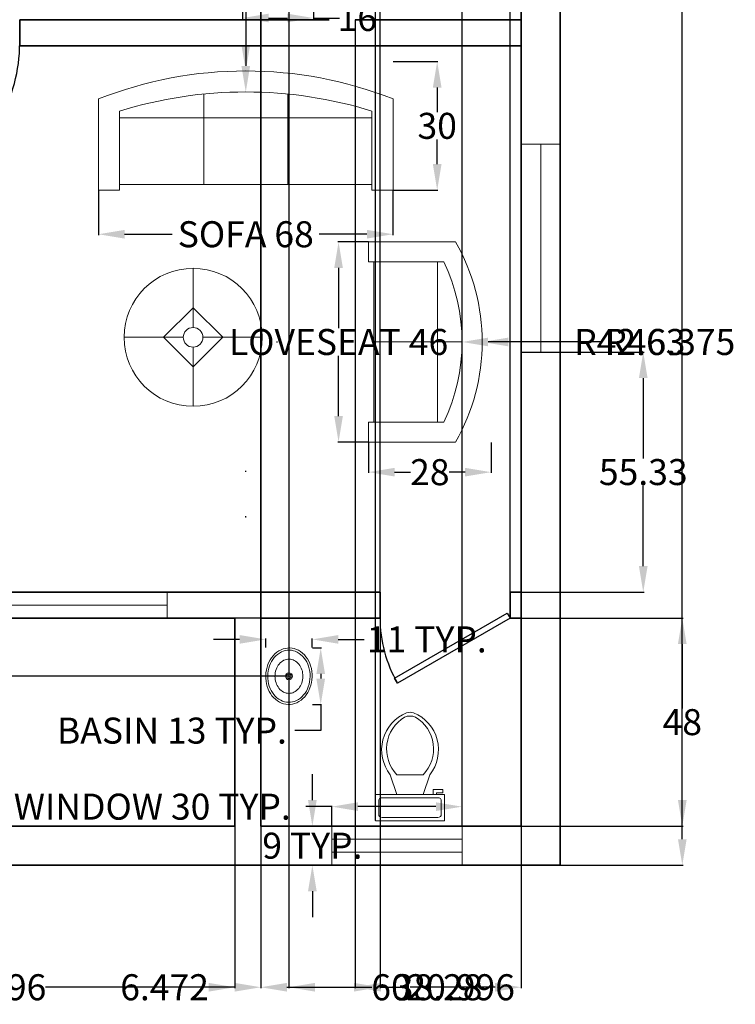
# Model space of a CAD drawing. Units: inches. Extents: x 351 to 774, y 111 to 703.
# Tile 3 of 6: x 608 to 773, y 111 to 338. Entities that reach past the tile are written whole.
import ezdxf

# ---------------------------------------------------------------- set-up
doc = ezdxf.new("R2010")
doc.units = ezdxf.units.IN
doc.header["$MEASUREMENT"] = 0
for name, color, linetype, lineweight in [('A-ANNO-DIMS', 2, 'Continuous', 18), ('A-DOOR', 3, 'Continuous', 25), ('A-FLOR-FIXT', 9, 'Continuous', 18), ('A-FURN', 8, 'Continuous', 18), ('A-GLAZ', 4, 'Continuous', 18), ('A-WALL', 7, 'Continuous', 35)]:
    doc.layers.add(name, color=color, linetype=linetype, lineweight=lineweight)
doc.styles.get("Standard").update_dxf_attribs({"font": 'arial.ttf'})
doc.dimstyles.get("Standard").update_dxf_attribs({"dimtxt": 6, "dimasz": 6, "dimexe": 0.18, "dimexo": 0.0625, "dimgap": 0.09, "dimtad": 0, "dimtih": 1, "dimtoh": 1, "dimdec": 0, "dimzin": 0, "dimdsep": 46, "dimlunit": 3, "dimtxsty": 'Standard', "dimcen": 0.09, "dimadec": 0, "dimazin": 0, "dimtfac": 1, "dimtdec": 0, "dimtofl": 0, "dimtmove": 0, "dimatfit": 3, "dimfxl": 1, "dimtolj": 1, "dimtzin": 0, "dimarcsym": 0})

# ---------------------------------------------------------------- blocks, each defined once
blk = doc.blocks.new('*U2')
for p, q in [((-40, 0), (-40, 6)), ((0, 0), (0, 6))]:
    blk.add_line(p, q)
blk.add_lwpolyline([(0, 0), (-34.64, -20), (-35.52, -18.48), (-0.88, 1.52)], close=True)
blk.add_arc((0, 0), 40, 180, 210)
blk = doc.blocks.new('*U5')
for p, q in [((0, 0), (0, 6)), ((40, 0), (40, 6))]:
    blk.add_line(p, q)
blk.add_lwpolyline([(0, 0), (34.64, -20), (35.52, -18.48), (0.88, 1.52)], close=True)
blk.add_arc((0, 0), 40, 330, 0)
blk = doc.blocks.new('Lamp - Table')
for p, q in [((0, 7), (0, 1)), ((0, 3), (-3, 0)), ((3, 0), (0, 3)), ((-1, 0), (-7, 0)), ((-3, 0), (0, -3)), ((0, -3), (3, 0)), ((1, 0), (7, 0)), ((0, -1), (0, -7))]:
    blk.add_line(p, q)
for radius in [7, 1]:
    blk.add_circle((0, 0), radius)
blk = doc.blocks.new('Sink - Oval top')
for p, q in [((-1, 0), (1, 0)), ((0, 1), (0, -1))]:
    blk.add_line(p, q)
for points in [[(-12.23, 0.39, 0.117634), (-11.46, -3.36, 0.104469), (-8.88, -6.8, 0.090016), (-5.08, -9.07, 0.08192), (-0.32, -10.02, 0.08192), (4.49, -9.38, 0.090016), (8.42, -7.36, 0.104469), (11.22, -4.09, 0.117634), (12.23, -0.39, 0.117634), (11.46, 3.36, 0.104469), (8.88, 6.8, 0.090016), (5.08, 9.07, 0.08192), (0.32, 10.02, 0.08192), (-4.49, 9.38, 0.090016), (-8.42, 7.36, 0.104469), (-11.22, 4.09, 0.117634)], [(-11.29, 0.16, 0.118622), (-10.52, -3.25, 0.104678), (-8.07, -6.36, 0.089562), (-4.54, -8.37, 0.081185), (-0.13, -9.15, 0.081185), (4.3, -8.49, 0.089562), (7.89, -6.58, 0.104678), (10.42, -3.55, 0.118622), (11.29, -0.16, 0.118622), (10.52, 3.25, 0.104678), (8.07, 6.36, 0.089562), (4.54, 8.37, 0.081185), (0.13, 9.15, 0.081185), (-4.3, 8.49, 0.089562), (-7.89, 6.58, 0.104678), (-10.42, 3.55, 0.118622)], [(-7.42, 0.08, 0.118283), (-6.91, -2.17, 0.104607), (-5.29, -4.21, 0.089718), (-2.97, -5.53, 0.081436), (-0.07, -6.04, 0.081436), (2.84, -5.59, 0.089718), (5.2, -4.33, 0.104607), (6.86, -2.32, 0.118283), (7.42, -0.08, 0.118283), (6.91, 2.17, 0.104607), (5.29, 4.21, 0.089718), (2.97, 5.53, 0.081436), (0.07, 6.04, 0.081436), (-2.84, 5.59, 0.089718), (-5.2, 4.33, 0.104607), (-6.86, 2.32, 0.118283)]]:
    blk.add_lwpolyline(points, format="xyb", close=True)
for radius in [1.5, 1]:
    blk.add_circle((0, 0), radius)
blk = doc.blocks.new('Sofa - Roundback 7 ft.')
for p, q in [((-12.00002, -32.4421), (-12.00003, -6.5971)), ((11.99997, -32.4421), (11.99998, -6.5971)), ((-36.000027, -34), (-36.000027, -11.4696)), ((-35.999844, -13.3819), (35.9998, -13.3819)), ((35.99998, -34), (35.99998, -11.4696)), ((-36.000027, -32.4421), (35.99998, -32.4421))]:
    blk.add_line(p, q)
for points in [[(-36.000027, -34), (-42.000027, -34), (-42.000027, -8)], [(41.99998, -8), (41.99998, -34), (35.99998, -34)]]:
    blk.add_lwpolyline(points)
for centre, radius, start, end in [((0, -114.25), 114.25, 68.43141, 111.5686), ((-0.00001, -127.1968), 121.1968, 72.72033, 107.2797)]:
    blk.add_arc(centre, radius, start, end)
blk = doc.blocks.new('Sofa - Roundback Loveseat 5 ft.')
for p, q in [((0, -32.44198), (0, -5.99998)), ((-24, -33.99998), (-24, -11.46958)), ((24.00004, -33.99998), (24.00004, -11.46958)), ((-23.9998, -13.38178), (23.99986, -13.38178)), ((-24, -32.44198), (24.00004, -32.44198))]:
    blk.add_line(p, q)
for points in [[(-24, -33.99998), (-30, -33.99998), (-30, -7.99998)], [(30.00004, -7.99998), (30.00004, -33.99998), (24.00004, -33.99998)]]:
    blk.add_lwpolyline(points)
for centre, radius, start, end in [((0, -60.24998), 60.24998, 60.13715, 119.8628), ((0, -61.38438), 55.38444, 64.32083, 115.6792)]:
    blk.add_arc(centre, radius, start, end)
blk = doc.blocks.new('Toilet - top')
for p, q in [((9.5, -6), (9.5, -2)), ((-10, -8.5), (-8, -8.5)), ((-10, -9.5), (-10, -8.5)), ((-8, -8.5), (-8, -8)), ((-7, -8), (-7, -9.5)), ((-4, -8), (-6, -14)), ((4, -8), (6, -14)), ((-7, -9.5), (-10, -9.5)), ((4, -14), (-4, -14))]:
    blk.add_line(p, q)
blk.add_lwpolyline([(10.5, -8), (10.5, 0), (-10.5, 0), (-10.5, -8)], close=True)
for points in [[(-9.5, -2), (-9.5, -6)], [(8.5, -1), (-8.5, -1)], [(-8.5, -7), (8.5, -7)]]:
    blk.add_lwpolyline(points)
for centre, radius, start, end in [((-8.62, -1.88), 0.884, 81.8699, 188.1301), ((8.62, -1.88), 0.884, 351.8699, 98.1301), ((-8.62, -6.12), 0.884, 171.8699, 278.1301), ((8.62, -6.12), 0.884, 261.8699, 8.1301), ((3.52, -21.58), 12.17, 141.4691, 247.9714), ((4.2, -21.82), 11.33, 136.3677, 238.9468), ((-3.52, -21.58), 12.17, 292.0284, 38.5307), ((-4.2, -21.82), 11.33, 301.053, 43.6321), ((0, -27.88), 4, 245.7318, 294.2682), ((0, -29), 4, 254.8605, 285.1395)]:
    blk.add_arc(centre, radius, start, end)
blk = doc.blocks.new('WIN-48IN-6IN-WALL')
blk.add_line((3, 48), (3, 0))
blk.add_lwpolyline([(0, 48), (6, 48), (6, 0), (0, 0)], close=True)
blk = doc.blocks.new('WIN-48IN-9IN-WALL')
blk.add_line((4.5, 48), (4.5, 0))
blk.add_lwpolyline([(0, 0), (9, 0), (9, 48), (0, 48)], close=True)
blk = doc.blocks.new('WIN-BATH-30IN-9IN-WALL')
for p, q in [((0, 0), (0, 9)), ((0, 9), (30, 9)), ((30, 9), (30, 0)), ((0, 6), (30, 6)), ((30, 3), (0, 3)), ((30, 0), (0, 0))]:
    blk.add_line(p, q)
blk = doc.blocks.new('*D26')
at = {"layer": 'A-ANNO-DIMS', "color": 0, "lineweight": -2, "transparency": 16777216}
for p, q in [((680.41, 156.74), (674.41, 156.74)), ((680.41, 152.3), (680.41, 156.92)), ((704.41, 156.74), (686.41, 156.74)), ((710.41, 152.3), (710.41, 156.92))]:
    blk.add_line(p, q, dxfattribs=at)
at = {"layer": 'A-ANNO-DIMS', "color": 0, "transparency": 16777216}
for points in [[(686.41, 157.74), (686.41, 155.74), (680.41, 156.74)], [(704.41, 157.74), (704.41, 155.74), (710.41, 156.74)]]:
    blk.add_solid(points, dxfattribs=at)
at = {"layer": 'Defpoints', "color": 0, "transparency": 16777216}
for p in [(680.41, 156.74), (680.41, 152.24), (710.41, 152.24)]:
    blk.add_point(p, dxfattribs=at)
at = {"layer": 'A-ANNO-DIMS', "color": 0, "transparency": 16777216, "insert": (631.89, 156.74), "char_height": 6, "attachment_point": 5}
blk.add_mtext('\\A1;WC WINDOW 30 TYP.', dxfattribs=at)
blk = doc.blocks.new('*D27')
at = {"layer": 'A-ANNO-DIMS', "color": 0, "lineweight": -2, "transparency": 16777216}
for p, q in [((675.91, 158.24), (675.91, 164.24)), ((680.35, 152.24), (675.73, 152.24)), ((680.35, 143.24), (675.73, 143.24)), ((675.91, 137.24), (675.91, 131.24))]:
    blk.add_line(p, q, dxfattribs=at)
at = {"layer": 'A-ANNO-DIMS', "color": 0, "transparency": 16777216}
for points in [[(674.91, 158.24), (676.91, 158.24), (675.91, 152.24)], [(674.91, 137.24), (676.91, 137.24), (675.91, 143.24)]]:
    blk.add_solid(points, dxfattribs=at)
at = {"layer": 'Defpoints', "color": 0, "transparency": 16777216}
for p in [(680.41, 152.24), (675.91, 143.24), (680.41, 143.24)]:
    blk.add_point(p, dxfattribs=at)
at = {"layer": 'A-ANNO-DIMS', "color": 0, "transparency": 16777216, "insert": (675.91, 147.74), "char_height": 6, "attachment_point": 5}
blk.add_mtext('\\A1;9 TYP.', dxfattribs=at)
blk = doc.blocks.new('*D30')
at = {"layer": 'A-ANNO-DIMS', "color": 0, "lineweight": -2, "transparency": 16777216}
for p, q in [((675.94, 193.36), (678.02, 193.36)), ((677.84, 187.36), (677.84, 186.28)), ((675.94, 180.28), (678.02, 180.28)), ((677.84, 180.28), (677.84, 174.28)), ((677.84, 174.28), (671.84, 174.28))]:
    blk.add_line(p, q, dxfattribs=at)
at = {"layer": 'A-ANNO-DIMS', "color": 0, "transparency": 16777216}
for points in [[(676.84, 187.36), (678.84, 187.36), (677.84, 193.36)], [(676.84, 186.28), (678.84, 186.28), (677.84, 180.28)]]:
    blk.add_solid(points, dxfattribs=at)
at = {"layer": 'Defpoints', "color": 0, "transparency": 16777216}
for p in [(675.88, 193.36), (675.88, 180.28), (677.84, 180.28)]:
    blk.add_point(p, dxfattribs=at)
at = {"layer": 'A-ANNO-DIMS', "color": 0, "transparency": 16777216, "insert": (643.54, 174.28), "char_height": 6, "attachment_point": 5}
blk.add_mtext('\\A1;BASIN 13 TYP.', dxfattribs=at)
blk = doc.blocks.new('*D31')
at = {"layer": 'A-ANNO-DIMS', "color": 0, "lineweight": -2, "transparency": 16777216}
for p, q in [((659.15, 195.32), (653.15, 195.32)), ((665.15, 193.42), (665.15, 195.5)), ((675.88, 193.42), (675.88, 195.5)), ((681.88, 195.32), (687.88, 195.32))]:
    blk.add_line(p, q, dxfattribs=at)
at = {"layer": 'A-ANNO-DIMS', "color": 0, "transparency": 16777216}
for points in [[(659.15, 196.32), (659.15, 194.32), (665.15, 195.32)], [(681.88, 196.32), (681.88, 194.32), (675.88, 195.32)]]:
    blk.add_solid(points, dxfattribs=at)
at = {"layer": 'Defpoints', "color": 0, "transparency": 16777216}
for p in [(675.88, 195.32), (665.15, 193.36), (675.88, 193.36)]:
    blk.add_point(p, dxfattribs=at)
at = {"layer": 'A-ANNO-DIMS', "color": 0, "transparency": 16777216, "insert": (702.29, 195.32), "char_height": 6, "attachment_point": 5}
blk.add_mtext('\\A1;11 TYP.', dxfattribs=at)
blk = doc.blocks.new('*D39')
at = {"layer": 'A-ANNO-DIMS', "color": 0, "lineweight": -2, "transparency": 16777216}
for p, q in [((659.83, 342.77), (659.83, 338.45)), ((676.17, 342.77), (676.17, 338.45)), ((665.83, 338.63), (670.17, 338.63)), ((676.17, 338.63), (682.17, 338.63))]:
    blk.add_line(p, q, dxfattribs=at)
at = {"layer": 'A-ANNO-DIMS', "color": 0, "transparency": 16777216}
for points in [[(665.83, 339.63), (665.83, 337.63), (659.83, 338.63)], [(670.17, 339.63), (670.17, 337.63), (676.17, 338.63)]]:
    blk.add_solid(points, dxfattribs=at)
at = {"layer": 'Defpoints', "color": 0, "transparency": 16777216}
for p in [(659.83, 342.83), (676.17, 342.83), (676.17, 338.63)]:
    blk.add_point(p, dxfattribs=at)
at = {"layer": 'A-ANNO-DIMS', "color": 0, "transparency": 16777216, "insert": (686.27, 338.63), "char_height": 6, "attachment_point": 5}
blk.add_mtext('\\A1;16', dxfattribs=at)
blk = doc.blocks.new('*D40')
at = {"layer": 'A-ANNO-DIMS', "color": 0, "lineweight": -2, "transparency": 16777216}
for p, q in [((626.61, 298.88), (626.61, 288.58)), ((694.5, 298.88), (694.5, 288.58)), ((632.61, 288.76), (643.6, 288.76)), ((688.5, 288.76), (677.51, 288.76))]:
    blk.add_line(p, q, dxfattribs=at)
at = {"layer": 'A-ANNO-DIMS', "color": 0, "transparency": 16777216}
for points in [[(632.61, 289.76), (632.61, 287.76), (626.61, 288.76)], [(688.5, 289.76), (688.5, 287.76), (694.5, 288.76)]]:
    blk.add_solid(points, dxfattribs=at)
at = {"layer": 'Defpoints', "color": 0, "transparency": 16777216}
for p in [(626.61, 298.94), (694.5, 298.94), (694.5, 288.76)]:
    blk.add_point(p, dxfattribs=at)
at = {"layer": 'A-ANNO-DIMS', "color": 0, "transparency": 16777216, "insert": (660.56, 288.76), "char_height": 6, "attachment_point": 5}
blk.add_mtext('\\A1;SOFA 68', dxfattribs=at)
blk = doc.blocks.new('*D41')
at = {"layer": 'A-ANNO-DIMS', "color": 0, "lineweight": -2, "transparency": 16777216}
for p, q in [((694.57, 328.58), (704.87, 328.58)), ((704.69, 322.58), (704.69, 316.92)), ((704.69, 304.94), (704.69, 310.61)), ((694.57, 298.94), (704.87, 298.94))]:
    blk.add_line(p, q, dxfattribs=at)
at = {"layer": 'A-ANNO-DIMS', "color": 0, "transparency": 16777216}
for points in [[(703.69, 322.58), (705.69, 322.58), (704.69, 328.58)], [(703.69, 304.94), (705.69, 304.94), (704.69, 298.94)]]:
    blk.add_solid(points, dxfattribs=at)
at = {"layer": 'Defpoints', "color": 0, "transparency": 16777216}
for p in [(694.5, 328.58), (704.69, 328.58), (694.5, 298.94)]:
    blk.add_point(p, dxfattribs=at)
at = {"layer": 'A-ANNO-DIMS', "color": 0, "transparency": 16777216, "insert": (704.69, 313.76), "char_height": 6, "attachment_point": 5}
blk.add_mtext('\\A1;30', dxfattribs=at)
blk = doc.blocks.new('*D42')
at = {"layer": 'A-ANNO-DIMS', "color": 0, "lineweight": -2, "transparency": 16777216}
for p, q in [((688.82, 287), (681.77, 287)), ((681.95, 281), (681.95, 267.1)), ((681.95, 246.82), (681.95, 260.71)), ((688.82, 240.82), (681.77, 240.82))]:
    blk.add_line(p, q, dxfattribs=at)
at = {"layer": 'A-ANNO-DIMS', "color": 0, "transparency": 16777216}
for points in [[(680.95, 281), (682.95, 281), (681.95, 287)], [(680.95, 246.82), (682.95, 246.82), (681.95, 240.82)]]:
    blk.add_solid(points, dxfattribs=at)
at = {"layer": 'Defpoints', "color": 0, "transparency": 16777216}
for p in [(688.88, 287), (681.95, 240.82), (688.88, 240.82)]:
    blk.add_point(p, dxfattribs=at)
at = {"layer": 'A-ANNO-DIMS', "color": 0, "transparency": 16777216, "insert": (681.95, 263.91), "char_height": 6, "attachment_point": 5}
blk.add_mtext('\\A1;LOVESEAT 46', dxfattribs=at)
blk = doc.blocks.new('*D43')
at = {"layer": 'A-ANNO-DIMS', "color": 0, "lineweight": -2, "transparency": 16777216}
for p, q in [((688.88, 240.75), (688.88, 233.71)), ((717.1, 240.75), (717.1, 233.71)), ((694.88, 233.89), (698.55, 233.89)), ((711.1, 233.89), (707.44, 233.89))]:
    blk.add_line(p, q, dxfattribs=at)
at = {"layer": 'A-ANNO-DIMS', "color": 0, "transparency": 16777216}
for points in [[(694.88, 234.89), (694.88, 232.89), (688.88, 233.89)], [(711.1, 234.89), (711.1, 232.89), (717.1, 233.89)]]:
    blk.add_solid(points, dxfattribs=at)
at = {"layer": 'Defpoints', "color": 0, "transparency": 16777216}
for p in [(688.88, 240.82), (717.1, 240.82), (717.1, 233.89)]:
    blk.add_point(p, dxfattribs=at)
at = {"layer": 'A-ANNO-DIMS', "color": 0, "transparency": 16777216, "insert": (702.99, 233.89), "char_height": 6, "attachment_point": 5}
blk.add_mtext('\\A1;28', dxfattribs=at)
blk = doc.blocks.new('*D47')
at = {"layer": 'A-ANNO-DIMS', "color": 0, "lineweight": -2, "transparency": 16777216}
for p, q in [((733.11, 671.24), (761.37, 671.24)), ((761.19, 665.24), (761.19, 410.4)), ((761.19, 149.24), (761.19, 404.09)), ((733.11, 143.24), (761.37, 143.24))]:
    blk.add_line(p, q, dxfattribs=at)
at = {"layer": 'A-ANNO-DIMS', "color": 0, "transparency": 16777216}
for points in [[(760.19, 665.24), (762.19, 665.24), (761.19, 671.24)], [(760.19, 149.24), (762.19, 149.24), (761.19, 143.24)]]:
    blk.add_solid(points, dxfattribs=at)
at = {"layer": 'Defpoints', "color": 0, "transparency": 16777216}
for p in [(733.04, 671.24), (761.19, 671.24), (733.04, 143.24)]:
    blk.add_point(p, dxfattribs=at)
at = {"layer": 'A-ANNO-DIMS', "color": 0, "transparency": 16777216, "insert": (761.19, 407.24), "char_height": 6, "attachment_point": 5}
blk.add_mtext('\\A1;528', dxfattribs=at)
blk = doc.blocks.new('*D61')
at = {"layer": 'A-ANNO-DIMS', "color": 0, "lineweight": -2, "transparency": 16777216}
for p, q in [((562.04, 152.18), (562.04, 114.91)), ((658.04, 152.18), (658.04, 114.91)), ((568.04, 115.09), (605.66, 115.09)), ((652.04, 115.09), (614.43, 115.09))]:
    blk.add_line(p, q, dxfattribs=at)
at = {"layer": 'A-ANNO-DIMS', "color": 0, "transparency": 16777216}
for points in [[(568.04, 116.09), (568.04, 114.09), (562.04, 115.09)], [(652.04, 116.09), (652.04, 114.09), (658.04, 115.09)]]:
    blk.add_solid(points, dxfattribs=at)
at = {"layer": 'Defpoints', "color": 0, "transparency": 16777216}
for p in [(562.04, 152.24), (658.04, 152.24), (658.04, 115.09)]:
    blk.add_point(p, dxfattribs=at)
at = {"layer": 'A-ANNO-DIMS', "color": 0, "transparency": 16777216, "insert": (610.04, 115.09), "char_height": 6, "attachment_point": 5}
blk.add_mtext('\\A1;96', dxfattribs=at)
blk = doc.blocks.new('*D62')
at = {"layer": 'A-ANNO-DIMS', "color": 0, "lineweight": -2, "transparency": 16777216}
for p, q in [((664.04, 152.18), (664.04, 114.91)), ((724.04, 152.18), (724.04, 114.91)), ((670.04, 115.09), (689.65, 115.09)), ((718.04, 115.09), (698.44, 115.09))]:
    blk.add_line(p, q, dxfattribs=at)
at = {"layer": 'A-ANNO-DIMS', "color": 0, "transparency": 16777216}
for points in [[(670.04, 116.09), (670.04, 114.09), (664.04, 115.09)], [(718.04, 116.09), (718.04, 114.09), (724.04, 115.09)]]:
    blk.add_solid(points, dxfattribs=at)
at = {"layer": 'Defpoints', "color": 0, "transparency": 16777216}
for p in [(664.04, 152.24), (724.04, 152.24), (724.04, 115.09)]:
    blk.add_point(p, dxfattribs=at)
at = {"layer": 'A-ANNO-DIMS', "color": 0, "transparency": 16777216, "insert": (694.04, 115.09), "char_height": 6, "attachment_point": 5}
blk.add_mtext('\\A1;60', dxfattribs=at)
blk = doc.blocks.new('*D63')
at = {"layer": 'A-ANNO-DIMS', "color": 0, "lineweight": -2, "transparency": 16777216}
for p, q in [((724.11, 200.24), (761.37, 200.24)), ((761.19, 194.24), (761.19, 179.4)), ((761.19, 158.24), (761.19, 173.09)), ((724.11, 152.24), (761.37, 152.24))]:
    blk.add_line(p, q, dxfattribs=at)
at = {"layer": 'A-ANNO-DIMS', "color": 0, "transparency": 16777216}
for points in [[(760.19, 194.24), (762.19, 194.24), (761.19, 200.24)], [(760.19, 158.24), (762.19, 158.24), (761.19, 152.24)]]:
    blk.add_solid(points, dxfattribs=at)
at = {"layer": 'Defpoints', "color": 0, "transparency": 16777216}
for p in [(724.04, 200.24), (761.19, 200.24), (724.04, 152.24)]:
    blk.add_point(p, dxfattribs=at)
at = {"layer": 'A-ANNO-DIMS', "color": 0, "transparency": 16777216, "insert": (761.19, 176.24), "char_height": 6, "attachment_point": 5}
blk.add_mtext('\\A1;48', dxfattribs=at)
blk = doc.blocks.new('*D67')
at = {"layer": 'A-ANNO-DIMS', "color": 0, "lineweight": -2, "transparency": 16777216}
for p, q in [((724.11, 261.57), (752.37, 261.57)), ((752.19, 255.57), (752.19, 237.06)), ((752.19, 212.24), (752.19, 230.75)), ((724.11, 206.24), (752.37, 206.24))]:
    blk.add_line(p, q, dxfattribs=at)
at = {"layer": 'A-ANNO-DIMS', "color": 0, "transparency": 16777216}
for points in [[(751.19, 255.57), (753.19, 255.57), (752.19, 261.57)], [(751.19, 212.24), (753.19, 212.24), (752.19, 206.24)]]:
    blk.add_solid(points, dxfattribs=at)
at = {"layer": 'Defpoints', "color": 0, "transparency": 16777216}
for p in [(724.04, 261.57), (724.04, 206.24), (752.19, 206.24)]:
    blk.add_point(p, dxfattribs=at)
at = {"layer": 'A-ANNO-DIMS', "color": 0, "transparency": 16777216, "insert": (752.19, 233.91), "char_height": 6, "attachment_point": 5}
blk.add_mtext('\\A1;55.33', dxfattribs=at)
blk = doc.blocks.new('*D68')
at = {"layer": 'A-ANNO-DIMS', "color": 0, "lineweight": -2, "transparency": 16777216}
for p, q in [((685.77, 338.18), (685.77, 114.91)), ((724.04, 338.18), (724.04, 114.91)), ((691.77, 115.09), (694.69, 115.09)), ((718.04, 115.09), (715.12, 115.09))]:
    blk.add_line(p, q, dxfattribs=at)
at = {"layer": 'A-ANNO-DIMS', "color": 0, "transparency": 16777216}
for points in [[(691.77, 116.09), (691.77, 114.09), (685.77, 115.09)], [(718.04, 116.09), (718.04, 114.09), (724.04, 115.09)]]:
    blk.add_solid(points, dxfattribs=at)
at = {"layer": 'Defpoints', "color": 0, "transparency": 16777216}
for p in [(685.77, 338.24), (724.04, 338.24), (724.04, 115.09)]:
    blk.add_point(p, dxfattribs=at)
at = {"layer": 'A-ANNO-DIMS', "color": 0, "transparency": 16777216, "insert": (704.9, 115.09), "char_height": 6, "attachment_point": 5}
blk.add_mtext('\\A1;38.28', dxfattribs=at)
blk = doc.blocks.new('*D69')
at = {"layer": 'A-ANNO-DIMS', "color": 0, "lineweight": -2, "transparency": 16777216}
for p, q in [((724.04, 473.44), (724.04, 114.91)), ((664.04, 470.18), (664.04, 114.91)), ((670.04, 115.09), (689.65, 115.09)), ((718.04, 115.09), (698.44, 115.09))]:
    blk.add_line(p, q, dxfattribs=at)
at = {"layer": 'A-ANNO-DIMS', "color": 0, "transparency": 16777216}
for points in [[(670.04, 116.09), (670.04, 114.09), (664.04, 115.09)], [(718.04, 116.09), (718.04, 114.09), (724.04, 115.09)]]:
    blk.add_solid(points, dxfattribs=at)
at = {"layer": 'Defpoints', "color": 0, "transparency": 16777216}
for p in [(724.04, 473.5), (664.04, 470.24), (724.04, 115.09)]:
    blk.add_point(p, dxfattribs=at)
at = {"layer": 'A-ANNO-DIMS', "color": 0, "transparency": 16777216, "insert": (694.04, 115.09), "char_height": 6, "attachment_point": 5}
blk.add_mtext('\\A1;60', dxfattribs=at)
blk = doc.blocks.new('*D86')
at = {"layer": 'A-ANNO-DIMS', "color": 0, "lineweight": -2, "transparency": 16777216}
for p, q in [((710.41, 152.3), (710.41, 699.57)), ((724.04, 152.3), (724.04, 699.57)), ((716.41, 699.39), (718.04, 699.39)), ((724.04, 699.39), (730.04, 699.39))]:
    blk.add_line(p, q, dxfattribs=at)
at = {"layer": 'A-ANNO-DIMS', "color": 0, "transparency": 16777216}
for points in [[(716.41, 700.39), (716.41, 698.39), (710.41, 699.39)], [(718.04, 700.39), (718.04, 698.39), (724.04, 699.39)]]:
    blk.add_solid(points, dxfattribs=at)
at = {"layer": 'Defpoints', "color": 0, "transparency": 16777216}
for p in [(724.04, 699.39), (710.41, 152.24), (724.04, 152.24)]:
    blk.add_point(p, dxfattribs=at)
at = {"layer": 'A-ANNO-DIMS', "color": 0, "transparency": 16777216, "insert": (742.3, 699.39), "char_height": 6, "attachment_point": 5}
blk.add_mtext('\\A1;13.633', dxfattribs=at)
blk = doc.blocks.new('*D87')
at = {"layer": 'A-ANNO-DIMS', "color": 0, "lineweight": -2, "transparency": 16777216}
for p, q in [((691.51, 206.3), (691.51, 699.57)), ((721.51, 206.3), (721.51, 699.57)), ((697.51, 699.39), (702.14, 699.39)), ((715.51, 699.39), (710.89, 699.39))]:
    blk.add_line(p, q, dxfattribs=at)
at = {"layer": 'A-ANNO-DIMS', "color": 0, "transparency": 16777216}
for points in [[(697.51, 700.39), (697.51, 698.39), (691.51, 699.39)], [(715.51, 700.39), (715.51, 698.39), (721.51, 699.39)]]:
    blk.add_solid(points, dxfattribs=at)
at = {"layer": 'Defpoints', "color": 0, "transparency": 16777216}
for p in [(721.51, 699.39), (691.51, 206.24), (721.51, 206.24)]:
    blk.add_point(p, dxfattribs=at)
at = {"layer": 'A-ANNO-DIMS', "color": 0, "transparency": 16777216, "insert": (706.51, 699.39), "char_height": 6, "attachment_point": 5}
blk.add_mtext('\\A1;30', dxfattribs=at)
blk = doc.blocks.new('*D88')
at = {"layer": 'A-ANNO-DIMS', "color": 0, "lineweight": -2, "transparency": 16777216}
for p, q in [((664.043027, 200.304576), (664.043027, 699.572076)), ((691.510725, 200.304576), (691.510725, 699.572076)), ((658.043027, 699.392076), (652.043027, 699.392076)), ((697.510725, 699.392076), (703.510725, 699.392076))]:
    blk.add_line(p, q, dxfattribs=at)
at = {"layer": 'A-ANNO-DIMS', "color": 0, "transparency": 16777216}
for points in [[(658.043027, 700.392076), (658.043027, 698.392076), (664.043027, 699.392076)], [(697.510725, 700.392076), (697.510725, 698.392076), (691.510725, 699.392076)]]:
    blk.add_solid(points, dxfattribs=at)
at = {"layer": 'Defpoints', "color": 0, "transparency": 16777216}
for p in [(691.510725, 699.392076), (664.043027, 200.242076), (691.510725, 200.242076)]:
    blk.add_point(p, dxfattribs=at)
at = {"layer": 'A-ANNO-DIMS', "color": 0, "transparency": 16777216, "insert": (677.776876, 699.392076), "char_height": 6, "attachment_point": 5}
blk.add_mtext('\\A1;27.47', dxfattribs=at)
blk = doc.blocks.new('*D101')
at = {"layer": 'A-ANNO-DIMS', "color": 0, "lineweight": -2, "transparency": 16777216}
for p, q in [((664.04, 152.3), (664.04, 699.57)), ((690.48, 153.55), (690.48, 699.57)), ((658.04, 699.39), (652.04, 699.39)), ((696.48, 699.39), (702.48, 699.39))]:
    blk.add_line(p, q, dxfattribs=at)
at = {"layer": 'A-ANNO-DIMS', "color": 0, "transparency": 16777216}
for points in [[(658.04, 700.39), (658.04, 698.39), (664.04, 699.39)], [(696.48, 700.39), (696.48, 698.39), (690.48, 699.39)]]:
    blk.add_solid(points, dxfattribs=at)
at = {"layer": 'Defpoints', "color": 0, "transparency": 16777216}
for p in [(664.04, 699.39), (664.04, 152.24), (690.48, 153.49)]:
    blk.add_point(p, dxfattribs=at)
at = {"layer": 'A-ANNO-DIMS', "color": 0, "transparency": 16777216, "insert": (677.26, 699.39), "char_height": 6, "attachment_point": 5}
blk.add_mtext('\\A1;26.433', dxfattribs=at)
blk = doc.blocks.new('*D102')
at = {"layer": 'A-ANNO-DIMS', "color": 0, "lineweight": -2, "transparency": 16777216}
for p, q in [((392.89, 200.24), (392.89, 206.24)), ((392.89, 206.24), (398.89, 206.24)), ((663.98, 200.24), (392.71, 200.24)), ((392.89, 192.82), (392.89, 194.24)), ((670.45, 186.82), (392.71, 186.82))]:
    blk.add_line(p, q, dxfattribs=at)
at = {"layer": 'A-ANNO-DIMS', "color": 0, "transparency": 16777216}
for points in [[(391.89, 194.24), (393.89, 194.24), (392.89, 200.24)], [(391.89, 192.82), (393.89, 192.82), (392.89, 186.82)]]:
    blk.add_solid(points, dxfattribs=at)
at = {"layer": 'Defpoints', "color": 0, "transparency": 16777216}
for p in [(392.89, 200.24), (664.04, 200.24), (670.51, 186.82)]:
    blk.add_point(p, dxfattribs=at)
at = {"layer": 'A-ANNO-DIMS', "color": 0, "transparency": 16777216, "insert": (411.14, 206.24), "char_height": 6, "attachment_point": 5}
blk.add_mtext('\\A1;13.424', dxfattribs=at)
blk = doc.blocks.new('*D108')
at = {"layer": 'A-ANNO-DIMS', "color": 0, "lineweight": -2, "transparency": 16777216}
for p, q in [((664.04, 527.44), (664.04, 114.91)), ((670.51, 515.76), (670.51, 114.91)), ((658.04, 115.09), (652.04, 115.09)), ((676.51, 115.09), (682.51, 115.09))]:
    blk.add_line(p, q, dxfattribs=at)
at = {"layer": 'A-ANNO-DIMS', "color": 0, "transparency": 16777216}
for points in [[(658.04, 116.09), (658.04, 114.09), (664.04, 115.09)], [(676.51, 116.09), (676.51, 114.09), (670.51, 115.09)]]:
    blk.add_solid(points, dxfattribs=at)
at = {"layer": 'Defpoints', "color": 0, "transparency": 16777216}
for p in [(664.04, 527.5), (670.51, 515.82), (664.04, 115.09)]:
    blk.add_point(p, dxfattribs=at)
at = {"layer": 'A-ANNO-DIMS', "color": 0, "transparency": 16777216, "insert": (641.84, 115.09), "char_height": 6, "attachment_point": 5}
blk.add_mtext('\\A1;6.472', dxfattribs=at)
blk = doc.blocks.new('*D109')
at = {"layer": 'A-ANNO-DIMS', "color": 0, "lineweight": -2, "transparency": 16777216}
for p, q in [((691.51, 200.18), (691.51, 114.91)), ((670.51, 186.76), (670.51, 114.91)), ((676.51, 115.09), (685.51, 115.09)), ((691.51, 115.09), (697.51, 115.09))]:
    blk.add_line(p, q, dxfattribs=at)
at = {"layer": 'A-ANNO-DIMS', "color": 0, "transparency": 16777216}
for points in [[(676.51, 116.09), (676.51, 114.09), (670.51, 115.09)], [(685.51, 116.09), (685.51, 114.09), (691.51, 115.09)]]:
    blk.add_solid(points, dxfattribs=at)
at = {"layer": 'Defpoints', "color": 0, "transparency": 16777216}
for p in [(691.51, 200.24), (670.51, 186.82), (691.51, 115.09)]:
    blk.add_point(p, dxfattribs=at)
at = {"layer": 'A-ANNO-DIMS', "color": 0, "transparency": 16777216, "insert": (710.1, 115.09), "char_height": 6, "attachment_point": 5}
blk.add_mtext('\\A1;20.996', dxfattribs=at)
blk = doc.blocks.new('*D110')
at = {"layer": 'A-ANNO-DIMS', "color": 0, "lineweight": -2, "transparency": 16777216}
for p, q in [((666.56, 380.35), (660.56, 380.35)), ((660.56, 380.35), (660.56, 327.58)), ((660.47, 223.61), (660.65, 223.61)), ((660.56, 223.52), (660.56, 223.7))]:
    blk.add_line(p, q, dxfattribs=at)
at = {"layer": 'A-ANNO-DIMS', "color": 0, "transparency": 16777216}
blk.add_solid([(659.56, 327.58), (661.56, 327.58), (660.56, 321.58)], dxfattribs=at)
at = {"layer": 'Defpoints', "color": 0, "transparency": 16777216}
for p in [(660.56, 321.58), (660.56, 223.61)]:
    blk.add_point(p, dxfattribs=at)
at = {"layer": 'A-ANNO-DIMS', "color": 0, "transparency": 16777216, "insert": (679.64, 380.35), "char_height": 6, "attachment_point": 5}
blk.add_mtext('\\A1;R97.96', dxfattribs=at)
blk = doc.blocks.new('*D111')
at = {"layer": 'A-ANNO-DIMS', "color": 0, "lineweight": -2, "transparency": 16777216}
for p, q in [((666.56, 381.83), (660.56, 381.83)), ((660.56, 381.83), (660.56, 332.43)), ((660.47, 234.08), (660.65, 234.08)), ((660.56, 233.99), (660.56, 234.17))]:
    blk.add_line(p, q, dxfattribs=at)
at = {"layer": 'A-ANNO-DIMS', "color": 0, "transparency": 16777216}
blk.add_solid([(659.56, 332.43), (661.56, 332.43), (660.56, 326.43)], dxfattribs=at)
at = {"layer": 'Defpoints', "color": 0, "transparency": 16777216}
for p in [(660.56, 326.43), (660.56, 234.08)]:
    blk.add_point(p, dxfattribs=at)
at = {"layer": 'A-ANNO-DIMS', "color": 0, "transparency": 16777216, "insert": (679.66, 381.83), "char_height": 6, "attachment_point": 5}
blk.add_mtext('\\A1;R92.35', dxfattribs=at)
blk = doc.blocks.new('*D112')
at = {"layer": 'A-ANNO-DIMS', "color": 0, "lineweight": -2, "transparency": 16777216}
for p, q in [((668.59, 263.91), (668.77, 263.91)), ((668.68, 263.82), (668.68, 264)), ((742.88, 263.91), (721.05, 263.91))]:
    blk.add_line(p, q, dxfattribs=at)
at = {"layer": 'A-ANNO-DIMS', "color": 0, "transparency": 16777216}
blk.add_solid([(721.05, 264.91), (721.05, 262.91), (715.05, 263.91)], dxfattribs=at)
at = {"layer": 'Defpoints', "color": 0, "transparency": 16777216}
for p in [(668.68, 263.91), (715.05, 263.91)]:
    blk.add_point(p, dxfattribs=at)
at = {"layer": 'A-ANNO-DIMS', "color": 0, "transparency": 16777216, "insert": (758.31, 263.91), "char_height": 6, "attachment_point": 5}
blk.add_mtext('\\A1;R46.375', dxfattribs=at)
blk = doc.blocks.new('*D113')
at = {"layer": 'A-ANNO-DIMS', "color": 0, "lineweight": -2, "transparency": 16777216}
for p, q in [((667.71, 263.91), (667.89, 263.91)), ((667.8, 263.82), (667.8, 264)), ((736.01, 263.91), (716.43, 263.91))]:
    blk.add_line(p, q, dxfattribs=at)
at = {"layer": 'A-ANNO-DIMS', "color": 0, "transparency": 16777216}
blk.add_solid([(716.43, 264.91), (716.43, 262.91), (710.43, 263.91)], dxfattribs=at)
at = {"layer": 'Defpoints', "color": 0, "transparency": 16777216}
for p in [(667.8, 263.91), (710.43, 263.91)]:
    blk.add_point(p, dxfattribs=at)
at = {"layer": 'A-ANNO-DIMS', "color": 0, "transparency": 16777216, "insert": (749.1, 263.91), "char_height": 6, "attachment_point": 5}
blk.add_mtext('\\A1;R42.63', dxfattribs=at)

msp = doc.modelspace()

# ---------------------------------------------------------------- linework, layer by layer
at = {"layer": 'A-WALL'}
for p, q in [((608.4474, 332.2421), (608.4474, 338.2421)), ((679.7664, 338.2421), (608.4474, 338.2421)), ((724.043, 338.2421), (685.7664, 338.2421)), ((724.043, 332.2421), (608.4474, 332.2421)), ((724.043, 332.2421), (724.043, 206.2421)), ((691.5107, 206.2421), (568.043, 206.2421)), ((724.043, 206.2421), (721.5107, 206.2421)), ((658.043, 200.2421), (562.043, 200.2421)), ((658.043, 200.2421), (658.043, 152.2421)), ((664.043, 200.2421), (664.043, 152.2421)), ((691.5107, 200.2421), (664.043, 200.2421)), ((724.043, 200.2421), (721.5107, 200.2421)), ((724.043, 200.2421), (724.043, 152.2421)), ((658.043, 152.2421), (562.043, 152.2421)), ((724.043, 152.2421), (664.043, 152.2421))]:
    msp.add_line(p, q, dxfattribs=at)
for points in [[(436.7781, 143.2421), (421.043, 143.2421), (421.043, 671.2421), (733.043, 671.2421), (733.043, 143.2421), (562.043, 143.2421)], [(691.5107, 206.2421), (691.5107, 200.2421)], [(721.5107, 200.2421), (721.5107, 206.2421)]]:
    msp.add_lwpolyline(points, dxfattribs=at)

# ---------------------------------------------------------------- block references
at = {"layer": 'A-DOOR'}
for name, p, xscale, yscale, zscale in [('*U5', (572.4474, 332.8421), 0.8999999999999985, 0.8999999999999985, 0.8999999999999985), ('*U2', (721.5107, 200.2421), 0.75, 0.75, 0.75)]:
    msp.add_blockref(name, p, dxfattribs=dict(at, xscale=xscale, yscale=yscale, zscale=zscale))
at = {"layer": 'A-FLOR-FIXT'}
for name, p, xscale, yscale, zscale, rotation in [('Sink - Oval top', (670.5147, 186.8184), 0.53295403104476, 0.53295403104476, 0.53295403104476, 270), ('Toilet - top', (698.432, 153.4918), 0.7577391478424742, 0.7577391478424742, 0.7577391478424742, 180)]:
    msp.add_blockref(name, p, dxfattribs=dict(at, xscale=xscale, yscale=yscale, zscale=zscale, rotation=rotation))
at = {"layer": 'A-FURN'}
for name, p, xscale, yscale, zscale in [('Sofa - Roundback 7 ft.', (660.5567, 326.4263), 0.808289947691827, 0.808289947691827, 0.808289947691827), ('Lamp - Table', (648.4198, 264.9833), 2.273403864676251, 2.273403864676251, 2.273403864676251)]:
    msp.add_blockref(name, p, dxfattribs=dict(at, xscale=xscale, yscale=yscale, zscale=zscale))
at = {"layer": 'A-FURN', "xscale": 0.7697116004593764, "yscale": 0.7697116004593764, "zscale": 0.7697116004593764, "rotation": 270}
msp.add_blockref('Sofa - Roundback Loveseat 5 ft.', (715.0514, 263.9087), dxfattribs=at)
at = {"layer": 'A-GLAZ'}
msp.add_blockref('WIN-48IN-9IN-WALL', (724.043, 261.5708), dxfattribs=at)
for name, p, rotation in [('WIN-48IN-6IN-WALL', (642.4563, 200.2421), 90.00000000000006), ('WIN-BATH-30IN-9IN-WALL', (710.4102, 152.2421), 180)]:
    msp.add_blockref(name, p, dxfattribs=dict(at, rotation=rotation))

# ---------------------------------------------------------------- dimensions: what is measured, and where the dimension line sits
at = {"layer": 'A-ANNO-DIMS'}
for base, p1, p2, override, picture, middle in [((691.5107, 699.3921), (664.043, 200.2421), (691.5107, 200.2421), {"dimdec": 2, "dimlfac": 1, "dimrnd": 0, "dimzin": 0, "dimdsep": 46, "dimlunit": 2}, '*D88', (677.7769, 699.3921)), ((664.043, 699.3921), (690.4757, 153.4918), (664.043, 152.2421), {"dimdec": 3, "dimlfac": 1, "dimrnd": 0, "dimzin": 0, "dimdsep": 46, "dimlunit": 2}, '*D101', (677.2594, 699.3921)), ((721.5107, 699.3921), (691.5107, 206.2421), (721.5107, 206.2421), {"dimdec": 0, "dimlfac": 1, "dimrnd": 0, "dimzin": 0, "dimdsep": 46, "dimlunit": 2}, '*D87', (706.5107, 699.3921)), ((724.043, 699.3921), (710.4102, 152.2421), (724.043, 152.2421), {"dimdec": 3, "dimlfac": 1, "dimrnd": 0, "dimzin": 0, "dimdsep": 46, "dimlunit": 2}, '*D86', (742.3049, 699.3921)), ((664.043, 115.0921), (670.5147, 515.8184), (664.043, 527.5), {"dimdec": 3, "dimlfac": 1, "dimrnd": 0, "dimzin": 0, "dimdsep": 46, "dimlunit": 2}, '*D108', (641.8439, 115.0921)), ((724.043, 115.0921), (664.043, 470.2421), (724.043, 473.5), {"dimdec": 0, "dimlfac": 1, "dimrnd": 0, "dimzin": 0, "dimdsep": 46, "dimlunit": 2}, '*D69', (694.043, 115.0921)), ((676.1667, 338.6333), (659.8333, 342.8333), (676.1667, 342.8333), {"dimdec": 0, "dimlfac": 1, "dimrnd": 0, "dimzin": 0, "dimdsep": 46, "dimlunit": 2}, '*D39', (686.2696, 338.6333)), ((724.043, 115.0921), (685.7664, 338.2421), (724.043, 338.2421), {"dimdec": 2, "dimlfac": 1, "dimrnd": 0, "dimzin": 0, "dimdsep": 46, "dimlunit": 2}, '*D68', (704.9047, 115.0921)), ((717.1039, 233.8899), (688.8812, 240.8173), (717.1039, 240.8173), {"dimdec": 0, "dimlfac": 1, "dimrnd": 0, "dimzin": 0, "dimdsep": 46, "dimlunit": 2}, '*D43', (702.9926, 233.8899)), ((691.5107, 115.0921), (670.5147, 186.8184), (691.5107, 200.2421), {"dimdec": 3, "dimlfac": 1, "dimrnd": 0, "dimzin": 0, "dimdsep": 46, "dimlunit": 2}, '*D109', (710.1041, 115.0921)), ((658.043, 115.0921), (562.043, 152.2421), (658.043, 152.2421), {"dimdec": 0, "dimlfac": 1, "dimrnd": 0, "dimzin": 0, "dimdsep": 46, "dimlunit": 2}, '*D61', (610.043, 115.0921)), ((724.043, 115.0921), (664.043, 152.2421), (724.043, 152.2421), {"dimdec": 0, "dimlfac": 1, "dimrnd": 0, "dimzin": 0, "dimdsep": 46, "dimlunit": 2}, '*D62', (694.043, 115.0921))]:
    dim = msp.add_linear_dim(base=base, p1=p1, p2=p2, dimstyle='Standard', override=override, dxfattribs=at)
    dim.commit()
    dim.dimension.update_dxf_attribs({"geometry": picture, "text_midpoint": middle})
for base, p1, p2, angle, override, picture, middle in [((761.193, 671.2421), (733.043, 143.2421), (733.043, 671.2421), 90, {"dimdec": 0, "dimlfac": 1, "dimrnd": 0, "dimzin": 0, "dimdsep": 46, "dimlunit": 2}, '*D47', (761.193, 407.2421)), ((704.6894, 328.5817), (694.5049, 298.9444), (694.5049, 328.5817), 90, {"dimdec": 0, "dimlfac": 1, "dimrnd": 0, "dimzin": 0, "dimdsep": 46, "dimlunit": 2}, '*D41', (704.6894, 313.763)), ((752.193, 206.2421), (724.043, 261.5708), (724.043, 206.2421), 270, {"dimdec": 2, "dimlfac": 1, "dimrnd": 0, "dimzin": 0, "dimdsep": 46, "dimlunit": 2}, '*D67', (752.193, 233.9064)), ((392.893, 200.2421), (670.5147, 186.8184), (664.043, 200.2421), 90, {"dimdec": 3, "dimlfac": 1, "dimrnd": 0, "dimzin": 0, "dimdsep": 46, "dimlunit": 2}, '*D102', (411.1426, 206.2421)), ((761.193, 200.2421), (724.043, 152.2421), (724.043, 200.2421), 90, {"dimdec": 0, "dimlfac": 1, "dimrnd": 0, "dimzin": 0, "dimdsep": 46, "dimlunit": 2}, '*D63', (761.193, 176.2421))]:
    dim = msp.add_linear_dim(base=base, p1=p1, p2=p2, angle=angle, dimstyle='Standard', override=override, dxfattribs=at)
    dim.commit()
    dim.dimension.update_dxf_attribs({"geometry": picture, "text_midpoint": middle})
for center, mpoint, override, picture, middle in [((660.5567, 234.0791), (660.557, 326.4263), {"dimdec": 2, "dimlfac": 1, "dimrnd": 0, "dimzin": 0, "dimdsep": 46, "dimlunit": 2}, '*D111', (679.6642, 381.8345)), ((660.5567, 223.6144), (660.557, 321.5765), {"dimdec": 2, "dimlfac": 1, "dimrnd": 0, "dimzin": 0, "dimdsep": 46, "dimlunit": 2}, '*D110', (679.6397, 380.3538)), ((667.8031, 263.9087), (710.4332, 263.909), {"dimdec": 2, "dimlfac": 1, "dimrnd": 0, "dimzin": 0, "dimdsep": 46, "dimlunit": 2}, '*D113', (736.0112, 263.9092)), ((668.6763, 263.9087), (715.0514, 263.909), {"dimdec": 3, "dimlfac": 1, "dimrnd": 0, "dimzin": 0, "dimdsep": 46, "dimlunit": 2}, '*D112', (742.8764, 263.9092))]:
    dim = msp.add_radius_dim(center=center, mpoint=mpoint, dimstyle='Standard', override=override, dxfattribs=at)
    dim.commit()
    dim.dimension.update_dxf_attribs({"geometry": picture, "text_midpoint": middle, "dimtype": 164})
for base, p1, p2, text, picture, middle in [((694.5049, 288.7599), (626.6085, 298.9444), (694.5049, 298.9444), 'SOFA <>', '*D40', (660.5567, 288.7599)), ((675.8807, 195.3233), (665.1488, 193.3607), (675.8807, 193.3607), '<> TYP.', '*D31', (702.2913, 195.3233))]:
    dim = msp.add_linear_dim(base=base, p1=p1, p2=p2, text=text, dimstyle='Standard', override={"dimdec": 0, "dimlfac": 1, "dimrnd": 0, "dimzin": 0, "dimdsep": 46, "dimlunit": 2}, dxfattribs=at)
    dim.commit()
    dim.dimension.update_dxf_attribs({"geometry": picture, "text_midpoint": middle})
for base, p1, p2, angle, text, picture, middle in [((681.9538, 240.8173), (688.8812, 287), (688.8812, 240.8173), 270, 'LOVESEAT <>', '*D42', (681.9538, 263.9086)), ((677.8434, 180.2762), (675.8807, 193.3607), (675.8807, 180.2762), 270, 'BASIN <> TYP.', '*D30', (643.5419, 174.2762)), ((680.4102, 156.7421), (710.4102, 152.2421), (680.4102, 152.2421), 180, 'WC WINDOW <> TYP.', '*D26', (631.8946, 156.7421)), ((675.9102, 143.2421), (680.4102, 152.2421), (680.4102, 143.2421), 270, '<> TYP.', '*D27', (675.9102, 147.7421))]:
    dim = msp.add_linear_dim(base=base, p1=p1, p2=p2, angle=angle, text=text, dimstyle='Standard', override={"dimdec": 0, "dimlfac": 1, "dimrnd": 0, "dimzin": 0, "dimdsep": 46, "dimlunit": 2}, dxfattribs=at)
    dim.commit()
    dim.dimension.update_dxf_attribs({"geometry": picture, "text_midpoint": middle})

doc.saveas('drawing.dxf')
